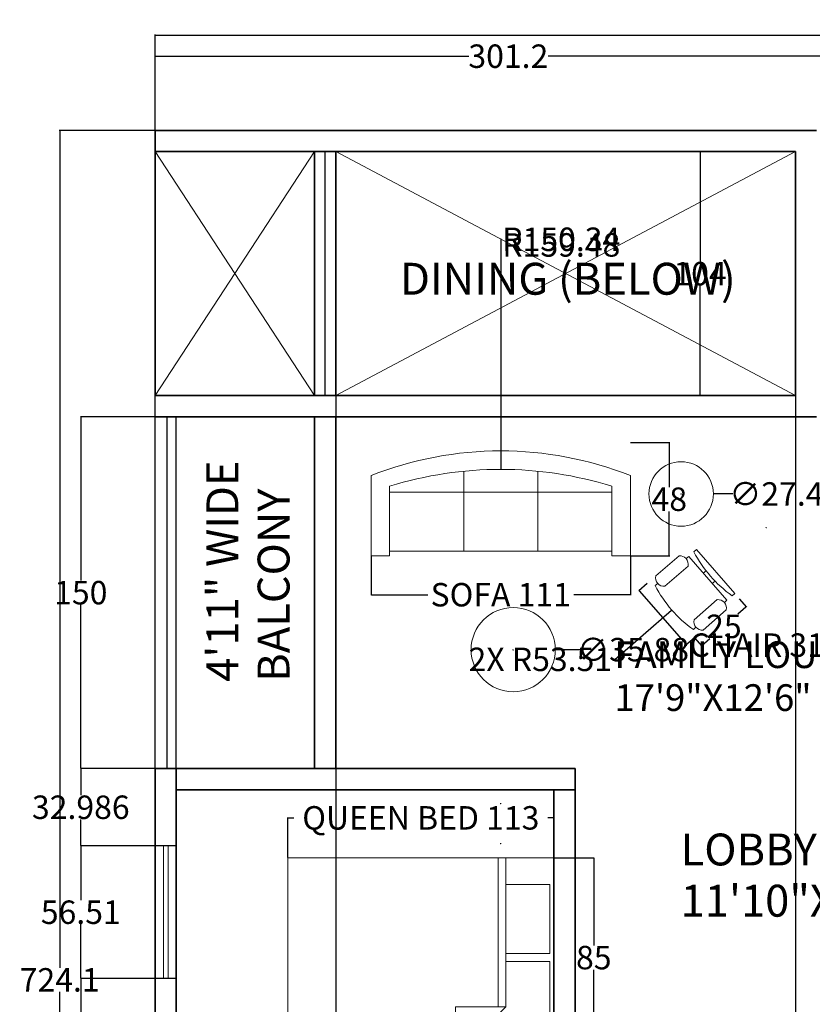
# Model space of a CAD drawing. Units: inches. Extents: x 135 to 880, y 60 to 879.
# Tile 4 of 5: x 135 to 473, y 459 to 879. Entities that reach past the tile are written whole.
import ezdxf

# ---------------------------------------------------------------- set-up
doc = ezdxf.new("R2010")
doc.units = ezdxf.units.IN
doc.header["$MEASUREMENT"] = 0
for name, color, linetype, lineweight in [('A-ANNO-DIMS', 2, 'Continuous', 18), ('A-AREA-IDEN', 7, 'Continuous', 18), ('A-FLOR-OPEN', 8, 'Continuous', 18), ('A-FLOR-RAIL', 8, 'Continuous', 25), ('A-FURN', 8, 'Continuous', 18), ('A-GLAZ', 4, 'Continuous', 18), ('A-WALL', 7, 'Continuous', 35)]:
    doc.layers.add(name, color=color, linetype=linetype, lineweight=lineweight)
doc.styles.get("Standard").update_dxf_attribs({"font": 'arial.ttf'})
doc.dimstyles.get("Standard").update_dxf_attribs({"dimtxt": 10, "dimasz": 0.18, "dimexe": 0.18, "dimexo": 0.0625, "dimgap": 0.09, "dimtad": 0, "dimtih": 1, "dimtoh": 1, "dimdec": 0, "dimzin": 0, "dimdsep": 46, "dimlunit": 3, "dimtxsty": 'Standard', "dimcen": 0.09, "dimadec": 0, "dimazin": 0, "dimtfac": 1, "dimtdec": 0, "dimtofl": 0, "dimtmove": 0, "dimatfit": 3, "dimfxl": 1, "dimtolj": 1, "dimtzin": 0, "dimarcsym": 0})

# ---------------------------------------------------------------- blocks, each defined once
blk = doc.blocks.new('Bed - Queen')
for p, q in [((0, -80.00003), (0, 0)), ((0, 0), (59.99999, 0)), ((59.99999, 0), (59.99999, -80.00003)), ((7.99999, -1.2), (28.79998, -1.2)), ((7.99999, -14.4), (7.99999, -1.2)), ((28.79998, -1.2), (28.79998, -14.4)), ((31.19999, -1.2), (51.99999, -1.2)), ((31.19999, -14.4), (31.19999, -1.2)), ((51.99999, -1.2), (51.99999, -16.4)), ((0, -14.4), (44.8, -14.4)), ((59.99999, -29.6), (44.8, -14.4)), ((44.8, -14.4), (44.8, -29.6)), ((44.8, -16.8), (0, -16.8)), ((51.99999, -16.4), (46.79936, -16.4)), ((44.8, -29.6), (59.99999, -29.6)), ((59.99999, -80.00003), (0, -80.00003))]:
    blk.add_line(p, q)
blk = doc.blocks.new('Sofa - Roundback 7 ft.')
for p, q in [((-12.00002, -32.4421), (-12.00003, -6.5971)), ((11.99997, -32.4421), (11.99998, -6.5971)), ((-36.000027, -34), (-36.000027, -11.4696)), ((35.99998, -34), (35.99998, -11.4696)), ((-35.999844, -13.3819), (35.9998, -13.3819)), ((-36.000027, -32.4421), (35.99998, -32.4421))]:
    blk.add_line(p, q)
for points in [[(-36.000027, -34), (-42.000027, -34), (-42.000027, -8)], [(41.99998, -8), (41.99998, -34), (35.99998, -34)]]:
    blk.add_lwpolyline(points)
for centre, radius, start, end in [((0, -114.25), 114.25, 68.43141, 111.5686), ((-0.00001, -127.1968), 121.1968, 72.72033, 107.2797)]:
    blk.add_arc(centre, radius, start, end)
blk = doc.blocks.new('Chair - Desk')
for p, q in [((-8.5, 0), (-8.5, -1)), ((-8.5, 0), (8.5, 0)), ((8.5, 0), (8.5, -1)), ((-2, -3), (-2, -1.9355)), ((2, -1.9576), (2, -3)), ((-10.5, -5), (-10.5, -14)), ((-8.5, -3), (-8.5, -4)), ((-8.5, -3), (8.5, -3)), ((-6.5, -14), (-6.5, -5)), ((6.5, -5), (6.5, -14)), ((8.5, -3), (8.5, -4)), ((10.5, -14), (10.5, -5)), ((-8.5, -15), (-8.5, -16)), ((8.5, -15), (8.5, -16))]:
    blk.add_line(p, q)
for centre, radius, start, end in [((0, 34.625), 36.625, 256.5803, 283.4197), ((-8.5, -6.5), 2.5, 36.8699, 143.1301), ((8.5, -6.5), 2.5, 36.8699, 143.1301), ((-8.5, -12.5), 2.5, 216.8699, 323.1301), ((8.5, -12.5), 2.5, 216.8699, 323.1301), ((0, 19.625), 36.625, 256.5803, 283.4197)]:
    blk.add_arc(centre, radius, start, end)
blk = doc.blocks.new('*D12')
at = {"layer": 'A-ANNO-DIMS', "color": 0, "lineweight": -2, "transparency": 16777216}
for p, q in [((402.69, 638.57), (399.13, 635.46)), ((399.38, 635.45), (419.31, 612.59)), ((422.85, 615.44), (419.29, 612.34)), ((419.42, 612.45), (419.54, 612.32)), ((419.54, 612.32), (419.72, 612.32))]:
    blk.add_line(p, q, dxfattribs=at)
at = {"layer": 'A-ANNO-DIMS', "color": 0, "transparency": 16777216}
for points in [[(399.41, 635.47), (399.36, 635.43), (399.27, 635.58)], [(419.33, 612.61), (419.28, 612.57), (419.42, 612.45)]]:
    blk.add_solid(points, dxfattribs=at)
at = {"layer": 'Defpoints', "color": 0, "transparency": 16777216}
for p in [(402.73, 638.61), (422.89, 615.48), (419.42, 612.45)]:
    blk.add_point(p, dxfattribs=at)
at = {"layer": 'A-ANNO-DIMS', "color": 0, "transparency": 16777216, "insert": (449.62, 612.32), "char_height": 10, "attachment_point": 5}
blk.add_mtext('\\A1;CHAIR 31', dxfattribs=at)
blk = doc.blocks.new('*D13')
at = {"layer": 'A-ANNO-DIMS', "color": 0, "lineweight": -2, "transparency": 16777216}
for p, q in [((442.02, 632.07), (445.13, 628.51)), ((444.87, 628.53), (441.42, 625.52)), ((422.93, 615.43), (426.03, 611.87)), ((426.05, 612.13), (429.5, 615.13))]:
    blk.add_line(p, q, dxfattribs=at)
at = {"layer": 'A-ANNO-DIMS', "color": 0, "transparency": 16777216}
for points in [[(444.85, 628.55), (444.89, 628.51), (445.01, 628.65)], [(426.03, 612.15), (426.07, 612.1), (425.92, 612.01)]]:
    blk.add_solid(points, dxfattribs=at)
at = {"layer": 'Defpoints', "color": 0, "transparency": 16777216}
for p in [(441.98, 632.12), (445.01, 628.65), (422.89, 615.48)]:
    blk.add_point(p, dxfattribs=at)
at = {"layer": 'A-ANNO-DIMS', "color": 0, "transparency": 16777216, "insert": (435.46, 620.33), "char_height": 10, "attachment_point": 5}
blk.add_mtext('\\A1;25', dxfattribs=at)
blk = doc.blocks.new('*D24')
at = {"layer": 'A-ANNO-DIMS', "color": 0, "lineweight": -2, "transparency": 16777216}
for p, q in [((249.52, 521.72), (249.52, 538.86)), ((249.7, 538.68), (252.04, 538.68)), ((362.8, 538.68), (360.46, 538.68)), ((362.98, 521.72), (362.98, 538.86))]:
    blk.add_line(p, q, dxfattribs=at)
at = {"layer": 'A-ANNO-DIMS', "color": 0, "transparency": 16777216}
for points in [[(249.7, 538.71), (249.7, 538.65), (249.52, 538.68)], [(362.8, 538.71), (362.8, 538.65), (362.98, 538.68)]]:
    blk.add_solid(points, dxfattribs=at)
at = {"layer": 'Defpoints', "color": 0, "transparency": 16777216}
for p in [(362.98, 538.68), (249.52, 521.66), (362.98, 521.66)]:
    blk.add_point(p, dxfattribs=at)
at = {"layer": 'A-ANNO-DIMS', "color": 0, "transparency": 16777216, "insert": (306.25, 538.68), "char_height": 10, "attachment_point": 5}
blk.add_mtext('\\A1;QUEEN BED 113', dxfattribs=at)
blk = doc.blocks.new('*D25')
at = {"layer": 'A-ANNO-DIMS', "color": 0, "lineweight": -2, "transparency": 16777216}
for p, q in [((363.04, 521.66), (380.17, 521.66)), ((379.99, 521.48), (379.99, 484.31)), ((379.99, 436.75), (379.99, 473.92)), ((363.04, 436.57), (380.17, 436.57))]:
    blk.add_line(p, q, dxfattribs=at)
at = {"layer": 'A-ANNO-DIMS', "color": 0, "transparency": 16777216}
for points in [[(379.96, 521.48), (380.02, 521.48), (379.99, 521.66)], [(379.96, 436.75), (380.02, 436.75), (379.99, 436.57)]]:
    blk.add_solid(points, dxfattribs=at)
at = {"layer": 'Defpoints', "color": 0, "transparency": 16777216}
for p in [(362.98, 521.66), (362.98, 436.57), (379.99, 436.57)]:
    blk.add_point(p, dxfattribs=at)
at = {"layer": 'A-ANNO-DIMS', "color": 0, "transparency": 16777216, "insert": (379.99, 479.12), "char_height": 10, "attachment_point": 5}
blk.add_mtext('\\A1;85', dxfattribs=at)
blk = doc.blocks.new('*D36')
at = {"layer": 'A-ANNO-DIMS', "color": 0, "lineweight": -2, "transparency": 16777216}
for p, q in [((285.05, 650.34), (285.05, 633.64)), ((395.59, 650.34), (395.59, 633.64)), ((285.23, 633.82), (309.21, 633.82)), ((395.41, 633.82), (371.43, 633.82))]:
    blk.add_line(p, q, dxfattribs=at)
at = {"layer": 'A-ANNO-DIMS', "color": 0, "transparency": 16777216}
for points in [[(285.23, 633.85), (285.23, 633.79), (285.05, 633.82)], [(395.41, 633.85), (395.41, 633.79), (395.59, 633.82)]]:
    blk.add_solid(points, dxfattribs=at)
at = {"layer": 'Defpoints', "color": 0, "transparency": 16777216}
for p in [(285.05, 650.4), (395.59, 650.4), (395.59, 633.82)]:
    blk.add_point(p, dxfattribs=at)
at = {"layer": 'A-ANNO-DIMS', "color": 0, "transparency": 16777216, "insert": (340.32, 633.82), "char_height": 10, "attachment_point": 5}
blk.add_mtext('\\A1;SOFA 111', dxfattribs=at)
blk = doc.blocks.new('*D37')
at = {"layer": 'A-ANNO-DIMS', "color": 0, "lineweight": -2, "transparency": 16777216}
for p, q in [((395.65, 698.65), (412.35, 698.65)), ((412.17, 698.47), (412.17, 679.72)), ((412.17, 650.58), (412.17, 669.33)), ((395.65, 650.4), (412.35, 650.4))]:
    blk.add_line(p, q, dxfattribs=at)
at = {"layer": 'A-ANNO-DIMS', "color": 0, "transparency": 16777216}
for points in [[(412.14, 698.47), (412.2, 698.47), (412.17, 698.65)], [(412.14, 650.58), (412.2, 650.58), (412.17, 650.4)]]:
    blk.add_solid(points, dxfattribs=at)
at = {"layer": 'Defpoints', "color": 0, "transparency": 16777216}
for p in [(395.59, 698.65), (412.17, 698.65), (395.59, 650.4)]:
    blk.add_point(p, dxfattribs=at)
at = {"layer": 'A-ANNO-DIMS', "color": 0, "transparency": 16777216, "insert": (412.17, 674.53), "char_height": 10, "attachment_point": 5}
blk.add_mtext('\\A1;48', dxfattribs=at)
blk = doc.blocks.new('*D38')
at = {"layer": 'A-ANNO-DIMS', "color": 0, "lineweight": -2, "transparency": 16777216}
for p, q in [((192.98, 831.76), (192.98, 872.58)), ((193.16, 872.4), (477.89, 872.4)), ((784.8, 872.4), (500.06, 872.4)), ((784.98, 831.76), (784.98, 872.58))]:
    blk.add_line(p, q, dxfattribs=at)
at = {"layer": 'A-ANNO-DIMS', "color": 0, "transparency": 16777216}
for points in [[(193.16, 872.43), (193.16, 872.37), (192.98, 872.4)], [(784.8, 872.43), (784.8, 872.37), (784.98, 872.4)]]:
    blk.add_solid(points, dxfattribs=at)
at = {"layer": 'Defpoints', "color": 0, "transparency": 16777216}
for p in [(784.98, 872.4), (192.98, 831.7), (784.98, 831.7)]:
    blk.add_point(p, dxfattribs=at)
at = {"layer": 'A-ANNO-DIMS', "color": 0, "transparency": 16777216, "insert": (488.98, 872.4), "char_height": 10, "attachment_point": 5}
blk.add_mtext('\\A1;592', dxfattribs=at)
blk = doc.blocks.new('*D39')
at = {"layer": 'A-ANNO-DIMS', "color": 0, "lineweight": -2, "transparency": 16777216}
for p, q in [((192.91, 831.7), (152.1, 831.7)), ((152.28, 831.52), (152.28, 474.74)), ((152.28, 107.73), (152.28, 464.52)), ((215.16, 107.55), (152.1, 107.55))]:
    blk.add_line(p, q, dxfattribs=at)
at = {"layer": 'A-ANNO-DIMS', "color": 0, "transparency": 16777216}
for points in [[(152.25, 831.52), (152.31, 831.52), (152.28, 831.7)], [(152.25, 107.73), (152.31, 107.73), (152.28, 107.55)]]:
    blk.add_solid(points, dxfattribs=at)
at = {"layer": 'Defpoints', "color": 0, "transparency": 16777216}
for p in [(152.28, 831.7), (192.98, 831.7), (215.22, 107.55)]:
    blk.add_point(p, dxfattribs=at)
at = {"layer": 'A-ANNO-DIMS', "color": 0, "transparency": 16777216, "insert": (152.28, 469.63), "char_height": 10, "attachment_point": 5}
blk.add_mtext('\\A1;724.1', dxfattribs=at)
blk = doc.blocks.new('*D40')
at = {"layer": 'A-ANNO-DIMS', "color": 0, "lineweight": -2, "transparency": 16777216}
for p, q in [((192.98, 822.76), (192.98, 863.58)), ((193.16, 863.4), (326.65, 863.4)), ((493.97, 863.4), (360.47, 863.4)), ((494.15, 822.76), (494.15, 863.58))]:
    blk.add_line(p, q, dxfattribs=at)
at = {"layer": 'A-ANNO-DIMS', "color": 0, "transparency": 16777216}
for points in [[(193.16, 863.43), (193.16, 863.37), (192.98, 863.4)], [(493.97, 863.43), (493.97, 863.37), (494.15, 863.4)]]:
    blk.add_solid(points, dxfattribs=at)
at = {"layer": 'Defpoints', "color": 0, "transparency": 16777216}
for p in [(494.15, 863.4), (192.98, 822.7), (494.15, 822.7)]:
    blk.add_point(p, dxfattribs=at)
at = {"layer": 'A-ANNO-DIMS', "color": 0, "transparency": 16777216, "insert": (343.56, 863.4), "char_height": 10, "attachment_point": 5}
blk.add_mtext('\\A1;301.2', dxfattribs=at)
blk = doc.blocks.new('*D50')
at = {"layer": 'A-ANNO-DIMS', "color": 0, "lineweight": -2, "transparency": 16777216}
for p, q in [((201.91, 470.2), (161.1, 470.2)), ((161.28, 470.02), (161.28, 435.15)), ((161.28, 389.88), (161.28, 424.76)), ((201.91, 389.7), (161.1, 389.7))]:
    blk.add_line(p, q, dxfattribs=at)
at = {"layer": 'A-ANNO-DIMS', "color": 0, "transparency": 16777216}
for points in [[(161.25, 470.02), (161.31, 470.02), (161.28, 470.2)], [(161.25, 389.88), (161.31, 389.88), (161.28, 389.7)]]:
    blk.add_solid(points, dxfattribs=at)
at = {"layer": 'Defpoints', "color": 0, "transparency": 16777216}
for p in [(161.28, 470.2), (201.98, 470.2), (201.98, 389.7)]:
    blk.add_point(p, dxfattribs=at)
at = {"layer": 'A-ANNO-DIMS', "color": 0, "transparency": 16777216, "insert": (161.28, 429.95), "char_height": 10, "attachment_point": 5}
blk.add_mtext('\\A1;80.5', dxfattribs=at)
blk = doc.blocks.new('*D51')
at = {"layer": 'A-ANNO-DIMS', "color": 0, "lineweight": -2, "transparency": 16777216}
for p, q in [((201.91, 526.72), (161.1, 526.72)), ((161.28, 526.54), (161.28, 503.65)), ((161.28, 470.38), (161.28, 493.26)), ((201.91, 470.2), (161.1, 470.2))]:
    blk.add_line(p, q, dxfattribs=at)
at = {"layer": 'A-ANNO-DIMS', "color": 0, "transparency": 16777216}
for points in [[(161.25, 526.54), (161.31, 526.54), (161.28, 526.72)], [(161.25, 470.38), (161.31, 470.38), (161.28, 470.2)]]:
    blk.add_solid(points, dxfattribs=at)
at = {"layer": 'Defpoints', "color": 0, "transparency": 16777216}
for p in [(161.28, 526.72), (201.98, 526.72), (201.98, 470.2)]:
    blk.add_point(p, dxfattribs=at)
at = {"layer": 'A-ANNO-DIMS', "color": 0, "transparency": 16777216, "insert": (161.28, 498.46), "char_height": 10, "attachment_point": 5}
blk.add_mtext('\\A1;56.51', dxfattribs=at)
blk = doc.blocks.new('*D52')
at = {"layer": 'A-ANNO-DIMS', "color": 0, "lineweight": -2, "transparency": 16777216}
for p, q in [((201.91, 559.7), (161.1, 559.7)), ((161.28, 559.52), (161.28, 548.41)), ((161.28, 526.9), (161.28, 538.01)), ((201.91, 526.72), (161.1, 526.72))]:
    blk.add_line(p, q, dxfattribs=at)
at = {"layer": 'A-ANNO-DIMS', "color": 0, "transparency": 16777216}
for points in [[(161.25, 559.52), (161.31, 559.52), (161.28, 559.7)], [(161.25, 526.9), (161.31, 526.9), (161.28, 526.72)]]:
    blk.add_solid(points, dxfattribs=at)
at = {"layer": 'Defpoints', "color": 0, "transparency": 16777216}
for p in [(161.28, 559.7), (201.98, 559.7), (201.98, 526.72)]:
    blk.add_point(p, dxfattribs=at)
at = {"layer": 'A-ANNO-DIMS', "color": 0, "transparency": 16777216, "insert": (161.28, 543.21), "char_height": 10, "attachment_point": 5}
blk.add_mtext('\\A1;32.986', dxfattribs=at)
blk = doc.blocks.new('*D53')
at = {"layer": 'A-ANNO-DIMS', "color": 0, "lineweight": -2, "transparency": 16777216}
for p, q in [((201.91, 709.7), (161.1, 709.7)), ((161.28, 709.52), (161.28, 639.9)), ((161.28, 559.88), (161.28, 629.51)), ((201.91, 559.7), (161.1, 559.7))]:
    blk.add_line(p, q, dxfattribs=at)
at = {"layer": 'A-ANNO-DIMS', "color": 0, "transparency": 16777216}
for points in [[(161.25, 709.52), (161.31, 709.52), (161.28, 709.7)], [(161.25, 559.88), (161.31, 559.88), (161.28, 559.7)]]:
    blk.add_solid(points, dxfattribs=at)
at = {"layer": 'Defpoints', "color": 0, "transparency": 16777216}
for p in [(161.28, 709.7), (201.98, 709.7), (201.98, 559.7)]:
    blk.add_point(p, dxfattribs=at)
at = {"layer": 'A-ANNO-DIMS', "color": 0, "transparency": 16777216, "insert": (161.28, 634.7), "char_height": 10, "attachment_point": 5}
blk.add_mtext('\\A1;150', dxfattribs=at)
blk = doc.blocks.new('*D72')
at = {"layer": 'A-ANNO-DIMS', "color": 0, "lineweight": -2, "transparency": 16777216}
for p, q in [((269.98, 822.64), (269.98, 66.67)), ((465.98, 822.64), (465.98, 66.67)), ((270.16, 66.85), (357.31, 66.85)), ((465.8, 66.85), (378.64, 66.85))]:
    blk.add_line(p, q, dxfattribs=at)
at = {"layer": 'A-ANNO-DIMS', "color": 0, "transparency": 16777216}
for points in [[(270.16, 66.88), (270.16, 66.82), (269.98, 66.85)], [(465.8, 66.88), (465.8, 66.82), (465.98, 66.85)]]:
    blk.add_solid(points, dxfattribs=at)
at = {"layer": 'Defpoints', "color": 0, "transparency": 16777216}
for p in [(269.98, 822.7), (465.98, 822.7), (465.98, 66.85)]:
    blk.add_point(p, dxfattribs=at)
at = {"layer": 'A-ANNO-DIMS', "color": 0, "transparency": 16777216, "insert": (367.98, 66.85), "char_height": 10, "attachment_point": 5}
blk.add_mtext('\\A1;196', dxfattribs=at)
blk = doc.blocks.new('*D73')
at = {"layer": 'A-ANNO-DIMS', "color": 0, "lineweight": -2, "transparency": 16777216}
for p, q in [((465.91, 822.7), (425.1, 822.7)), ((425.28, 822.52), (425.28, 775.9)), ((425.28, 718.88), (425.28, 765.51)), ((465.91, 718.7), (425.1, 718.7))]:
    blk.add_line(p, q, dxfattribs=at)
at = {"layer": 'A-ANNO-DIMS', "color": 0, "transparency": 16777216}
for points in [[(425.25, 822.52), (425.31, 822.52), (425.28, 822.7)], [(425.25, 718.88), (425.31, 718.88), (425.28, 718.7)]]:
    blk.add_solid(points, dxfattribs=at)
at = {"layer": 'Defpoints', "color": 0, "transparency": 16777216}
for p in [(425.28, 822.7), (465.98, 822.7), (465.98, 718.7)]:
    blk.add_point(p, dxfattribs=at)
at = {"layer": 'A-ANNO-DIMS', "color": 0, "transparency": 16777216, "insert": (425.28, 770.7), "char_height": 10, "attachment_point": 5}
blk.add_mtext('\\A1;104', dxfattribs=at)
blk = doc.blocks.new('*D79')
at = {"layer": 'A-ANNO-DIMS', "color": 0, "lineweight": -2, "transparency": 16777216}
for p, q in [((345.54, 610.39), (345.72, 610.39)), ((345.63, 610.3), (345.63, 610.48)), ((374.33, 610.39), (363.75, 610.39))]:
    blk.add_line(p, q, dxfattribs=at)
at = {"layer": 'A-ANNO-DIMS', "color": 0, "transparency": 16777216}
blk.add_solid([(363.75, 610.42), (363.75, 610.36), (363.57, 610.39)], dxfattribs=at)
at = {"layer": 'Defpoints', "color": 0, "transparency": 16777216}
for p in [(327.68, 610.39), (363.57, 610.39)]:
    blk.add_point(p, dxfattribs=at)
at = {"layer": 'A-ANNO-DIMS', "color": 0, "transparency": 16777216, "insert": (396.74, 610.39), "char_height": 10, "attachment_point": 5}
blk.add_mtext('\\A1;∅35.88', dxfattribs=at)
blk = doc.blocks.new('*D81')
at = {"layer": 'A-ANNO-DIMS', "color": 0, "lineweight": -2, "transparency": 16777216}
for p, q in [((417.13, 676.77), (417.31, 676.77)), ((417.22, 676.68), (417.22, 676.86)), ((439.22, 676.77), (431.15, 676.77))]:
    blk.add_line(p, q, dxfattribs=at)
at = {"layer": 'A-ANNO-DIMS', "color": 0, "transparency": 16777216}
blk.add_solid([(431.15, 676.8), (431.15, 676.74), (430.97, 676.77)], dxfattribs=at)
at = {"layer": 'Defpoints', "color": 0, "transparency": 16777216}
for p in [(403.48, 676.77), (430.97, 676.77)]:
    blk.add_point(p, dxfattribs=at)
at = {"layer": 'A-ANNO-DIMS', "color": 0, "transparency": 16777216, "insert": (461.63, 676.77), "char_height": 10, "attachment_point": 5}
blk.add_mtext('\\A1;∅27.49', dxfattribs=at)
blk = doc.blocks.new('*D83')
at = {"layer": 'A-ANNO-DIMS', "color": 0, "lineweight": -2, "transparency": 16777216}
for p, q in [((340.5, 782.94), (340.32, 782.94)), ((340.32, 782.94), (340.32, 687.43)), ((340.23, 527.77), (340.41, 527.77)), ((340.32, 527.68), (340.32, 527.86))]:
    blk.add_line(p, q, dxfattribs=at)
at = {"layer": 'A-ANNO-DIMS', "color": 0, "transparency": 16777216}
blk.add_solid([(340.29, 687.43), (340.35, 687.43), (340.32, 687.25)], dxfattribs=at)
at = {"layer": 'Defpoints', "color": 0, "transparency": 16777216}
for p in [(340.32, 687.25), (340.32, 527.77)]:
    blk.add_point(p, dxfattribs=at)
at = {"layer": 'A-ANNO-DIMS', "color": 0, "transparency": 16777216, "insert": (366.14, 782.94), "char_height": 10, "attachment_point": 5}
blk.add_mtext('\\A1;R159.48', dxfattribs=at)
blk = doc.blocks.new('*D84')
at = {"layer": 'A-ANNO-DIMS', "color": 0, "lineweight": -2, "transparency": 16777216}
for p, q in [((340.5, 785.35), (340.32, 785.35)), ((340.32, 785.35), (340.32, 695.32)), ((340.23, 544.8), (340.41, 544.8)), ((340.32, 544.71), (340.32, 544.89))]:
    blk.add_line(p, q, dxfattribs=at)
at = {"layer": 'A-ANNO-DIMS', "color": 0, "transparency": 16777216}
blk.add_solid([(340.29, 695.32), (340.35, 695.32), (340.32, 695.14)], dxfattribs=at)
at = {"layer": 'Defpoints', "color": 0, "transparency": 16777216}
for p in [(340.32, 695.14), (340.32, 544.8)]:
    blk.add_point(p, dxfattribs=at)
at = {"layer": 'A-ANNO-DIMS', "color": 0, "transparency": 16777216, "insert": (366.11, 785.35), "char_height": 10, "attachment_point": 5}
blk.add_mtext('\\A1;R150.34', dxfattribs=at)
blk = doc.blocks.new('*D87')
at = {"layer": 'A-ANNO-DIMS', "color": 0, "lineweight": -2, "transparency": 16777216}
for p, q in [((453.43, 662.52), (453.61, 662.52)), ((453.52, 662.43), (453.52, 662.61)), ((388.98, 606.27), (413.05, 627.24)), ((388.8, 606.27), (388.98, 606.27))]:
    blk.add_line(p, q, dxfattribs=at)
at = {"layer": 'A-ANNO-DIMS', "color": 0, "transparency": 16777216}
blk.add_solid([(413.03, 627.27), (413.07, 627.22), (413.18, 627.36)], dxfattribs=at)
at = {"layer": 'Defpoints', "color": 0, "transparency": 16777216}
for p in [(453.52, 662.52), (413.18, 627.36)]:
    blk.add_point(p, dxfattribs=at)
at = {"layer": 'A-ANNO-DIMS', "color": 0, "transparency": 16777216, "insert": (357.19, 606.27), "char_height": 10, "attachment_point": 5}
blk.add_mtext('\\A1;2X R53.51', dxfattribs=at)

msp = doc.modelspace()

# ---------------------------------------------------------------- linework, layer by layer
at = {"layer": 'A-FLOR-OPEN'}
for p, q in [((192.9753, 822.7014), (260.9753, 718.7014)), ((192.9753, 718.7014), (260.9753, 822.7014)), ((269.9753, 822.7014), (465.9753, 718.7014)), ((269.9753, 718.7014), (465.9753, 822.7014))]:
    msp.add_line(p, q, dxfattribs=at)
at = {"layer": 'A-FLOR-RAIL'}
for p, q in [((265.3866, 822.7014), (265.3866, 718.7014)), ((192.9753, 559.7014), (192.9753, 718.7014)), ((198.0257, 709.7014), (198.0257, 559.7014)), ((201.9753, 559.7014), (201.9753, 709.7014))]:
    msp.add_line(p, q, dxfattribs=at)
at = {"layer": 'A-FURN'}
for centre, radius in [((417.2227, 676.7728), 13.7453), ((345.6255, 610.3932), 17.9412)]:
    msp.add_circle(centre, radius, dxfattribs=at)
at = {"layer": 'A-GLAZ'}
for p, q in [((201.9753, 526.7153), (192.9753, 526.7153)), ((196.4753, 526.7153), (196.4753, 470.2014)), ((198.4753, 526.7153), (198.4753, 470.2014)), ((201.9753, 470.2014), (192.9753, 470.2014))]:
    msp.add_line(p, q, dxfattribs=at)
at = {"layer": 'A-WALL'}
for p, q in [((192.9753, 831.7014), (192.9753, 718.7014)), ((269.9753, 831.7014), (192.9753, 831.7014)), ((474.9753, 831.7014), (269.9753, 831.7014)), ((260.9753, 822.7014), (192.9753, 822.7014)), ((260.9753, 718.7014), (260.9753, 822.7014)), ((465.9753, 822.7014), (260.9753, 822.7014)), ((269.9753, 718.7014), (269.9753, 822.7014)), ((465.9753, 718.7014), (465.9753, 822.7014)), ((192.9753, 718.7014), (260.9753, 718.7014)), ((465.9753, 718.7014), (260.9753, 718.7014)), ((192.9753, 709.7014), (269.9753, 709.7014)), ((260.9753, 709.7014), (260.9753, 559.7014)), ((269.9753, 709.7014), (269.9753, 559.7014)), ((474.9753, 709.7014), (269.9753, 709.7014)), ((192.9753, 389.7014), (192.9753, 559.7014)), ((192.9753, 559.7014), (371.9753, 559.7014)), ((201.9753, 550.7014), (201.9753, 559.7014)), ((269.9753, 559.7014), (371.9753, 559.7014)), ((371.9753, 559.7014), (371.9753, 389.7014)), ((201.9753, 389.7014), (201.9753, 550.7014)), ((201.9753, 550.7014), (362.9753, 550.7014)), ((269.9753, 550.7014), (371.9753, 550.7014)), ((362.9753, 550.7014), (362.9753, 389.7014))]:
    msp.add_line(p, q, dxfattribs=at)

# ---------------------------------------------------------------- block references
at = {"layer": 'A-FURN', "xscale": 1.315875208097639, "yscale": 1.315875208097639, "zscale": 1.315875208097639}
msp.add_blockref('Sofa - Roundback 7 ft.', (340.3196, 695.1433), dxfattribs=at)
at = {"layer": 'A-FURN'}
for name, p, xscale, yscale, zscale, rotation in [('Chair - Desk', (431.9043, 643.6808), 1.46097776508805, 1.46097776508805, 1.46097776508805, 311.0737159505713), ('Bed - Queen', (362.9753, 521.6594), 1.418135637024811, 1.418135637024811, 1.418135637024811, 270)]:
    msp.add_blockref(name, p, dxfattribs=dict(at, xscale=xscale, yscale=yscale, zscale=zscale, rotation=rotation))

# ---------------------------------------------------------------- texts
at = {"layer": 'A-AREA-IDEN'}
for s, height, p in [('DINING (BELOW)', 13.591192, (297.3898, 761.7247)), ('FAMILY LOUNGE ', 11.388789, (388.8064, 602.5497)), ('17\'9"X12\'6"', 11.388789, (388.8064, 584.2546)), ('LOBBY', 13.59119, (417.0166, 518.4017)), ('11\'10"X13\'5"', 13.591192, (417.0166, 496.5687))]:
    msp.add_text(s, height=height, dxfattribs=at).set_placement(p)
for s, height, p in [('4\'11" WIDE ', 13.591192, (228.4366, 596.6914)), ('BALCONY ', 13.59119, (250.2696, 596.6914))]:
    msp.add_text(s, height=height, rotation=90, dxfattribs=at).set_placement(p)

# ---------------------------------------------------------------- dimensions: what is measured, and where the dimension line sits
at = {"layer": 'A-ANNO-DIMS'}
for base, p1, p2, override, picture, middle in [((784.9753, 872.4014), (192.9753, 831.7014), (784.9753, 831.7014), {"dimdec": 0, "dimlfac": 1, "dimrnd": 0, "dimzin": 0, "dimdsep": 46, "dimlunit": 2}, '*D38', (488.9753, 872.4014)), ((494.1454, 863.4014), (192.9753, 822.7014), (494.1454, 822.7014), {"dimdec": 1, "dimlfac": 1, "dimrnd": 0, "dimzin": 0, "dimdsep": 46, "dimlunit": 2}, '*D40', (343.5604, 863.4014)), ((465.9753, 66.853), (269.9753, 822.7014), (465.9753, 822.7014), {"dimdec": 0, "dimlfac": 1, "dimrnd": 0, "dimzin": 0, "dimdsep": 46, "dimlunit": 2}, '*D72', (367.9753, 66.853))]:
    dim = msp.add_linear_dim(base=base, p1=p1, p2=p2, dimstyle='Standard', override=override, dxfattribs=at)
    dim.commit()
    dim.dimension.update_dxf_attribs({"geometry": picture, "text_midpoint": middle})
for base, p1, p2, angle, override, picture, middle in [((152.2753, 831.7014), (215.2242, 107.553), (192.9753, 831.7014), 90, {"dimdec": 1, "dimlfac": 1, "dimrnd": 0, "dimzin": 0, "dimdsep": 46, "dimlunit": 2}, '*D39', (152.2753, 469.6272)), ((425.2753, 822.7014), (465.9753, 718.7014), (465.9753, 822.7014), 90, {"dimdec": 0, "dimlfac": 1, "dimrnd": 0, "dimzin": 0, "dimdsep": 46, "dimlunit": 2}, '*D73', (425.2753, 770.7014)), ((161.2753, 709.7014), (201.9753, 559.7014), (201.9753, 709.7014), 90, {"dimdec": 0, "dimlfac": 1, "dimrnd": 0, "dimzin": 0, "dimdsep": 46, "dimlunit": 2}, '*D53', (161.2753, 634.7014)), ((412.1664, 698.6523), (395.5864, 650.4036), (395.5864, 698.6523), 90, {"dimdec": 0, "dimlfac": 1, "dimrnd": 0, "dimzin": 0, "dimdsep": 46, "dimlunit": 2}, '*D37', (412.1664, 674.528)), ((445.007, 628.647), (422.8927, 615.478), (441.9833, 632.1163), 41.073716, {"dimdec": 0, "dimlfac": 1, "dimrnd": 0, "dimzin": 0, "dimdsep": 46, "dimlunit": 2}, '*D13', (435.4617, 620.3278)), ((161.2753, 559.7014), (201.9753, 526.7153), (201.9753, 559.7014), 90, {"dimdec": 3, "dimlfac": 1, "dimrnd": 0, "dimzin": 0, "dimdsep": 46, "dimlunit": 2}, '*D52', (161.2753, 543.2083)), ((161.2753, 526.7153), (201.9753, 470.2014), (201.9753, 526.7153), 90, {"dimdec": 2, "dimlfac": 1, "dimrnd": 0, "dimzin": 0, "dimdsep": 46, "dimlunit": 2}, '*D51', (161.2753, 498.4583)), ((379.993, 436.5713), (362.9753, 521.6594), (362.9753, 436.5713), 270, {"dimdec": 0, "dimlfac": 1, "dimrnd": 0, "dimzin": 0, "dimdsep": 46, "dimlunit": 2}, '*D25', (379.993, 479.1154)), ((161.2753, 470.2014), (201.9753, 389.7014), (201.9753, 470.2014), 90, {"dimdec": 1, "dimlfac": 1, "dimrnd": 0, "dimzin": 0, "dimdsep": 46, "dimlunit": 2}, '*D50', (161.2753, 429.9514))]:
    dim = msp.add_linear_dim(base=base, p1=p1, p2=p2, angle=angle, dimstyle='Standard', override=override, dxfattribs=at)
    dim.commit()
    dim.dimension.update_dxf_attribs({"geometry": picture, "text_midpoint": middle})
for center, mpoint, picture, middle in [((340.3196, 544.8046), (340.32, 695.1433), '*D84', (366.1121, 785.3466)), ((340.3196, 527.7682), (340.32, 687.2481), '*D83', (366.1428, 782.936))]:
    dim = msp.add_radius_dim(center=center, mpoint=mpoint, dimstyle='Standard', override={"dimdec": 2, "dimlfac": 1, "dimrnd": 0, "dimzin": 0, "dimdsep": 46, "dimlunit": 2}, dxfattribs=at)
    dim.commit()
    dim.dimension.update_dxf_attribs({"geometry": picture, "text_midpoint": middle, "dimtype": 164})
for p1, p2, picture, middle in [((403.4773, 676.7726), (430.968, 676.773), '*D81', (439.2152, 676.7731)), ((327.6843, 610.3934), (363.5666, 610.393), '*D79', (374.3314, 610.3929))]:
    dim = msp.add_diameter_dim_2p(p1=p1, p2=p2, dimstyle='Standard', override={"dimdec": 2, "dimlfac": 1, "dimrnd": 0, "dimzin": 0, "dimdsep": 46, "dimlunit": 2}, dxfattribs=at)
    dim.commit()
    dim.dimension.update_dxf_attribs({"geometry": picture, "text_midpoint": middle, "dimtype": 163})
dim = msp.add_radius_dim(center=(453.5188, 662.519), mpoint=(413.1811, 627.3621), text='2X <>', dimstyle='Standard', override={"dimdec": 2, "dimlfac": 1, "dimrnd": 0, "dimzin": 0, "dimdsep": 46, "dimlunit": 2}, dxfattribs=at)
dim.commit()
dim.dimension.update_dxf_attribs({"geometry": '*D87', "text_midpoint": (357.1873, 606.268), "dimtype": 164})
for base, p1, p2, text, picture, middle in [((395.5864, 633.8236), (285.0528, 650.4036), (395.5864, 650.4036), 'SOFA <>', '*D36', (340.3196, 633.8236)), ((362.9753, 538.6771), (249.5244, 521.6594), (362.9753, 521.6594), 'QUEEN BED <>', '*D24', (306.2499, 538.6771))]:
    dim = msp.add_linear_dim(base=base, p1=p1, p2=p2, text=text, dimstyle='Standard', override={"dimdec": 0, "dimlfac": 1, "dimrnd": 0, "dimzin": 0, "dimdsep": 46, "dimlunit": 2}, dxfattribs=at)
    dim.commit()
    dim.dimension.update_dxf_attribs({"geometry": picture, "text_midpoint": middle})
dim = msp.add_linear_dim(base=(419.4233, 612.4543), p1=(402.7347, 638.6069), p2=(422.8927, 615.478), angle=311.073716, text='CHAIR <>', dimstyle='Standard', override={"dimdec": 0, "dimlfac": 1, "dimrnd": 0, "dimzin": 0, "dimdsep": 46, "dimlunit": 2}, dxfattribs=at)
dim.commit()
dim.dimension.update_dxf_attribs({"geometry": '*D12', "text_midpoint": (449.624, 612.3186)})

doc.saveas('drawing.dxf')
